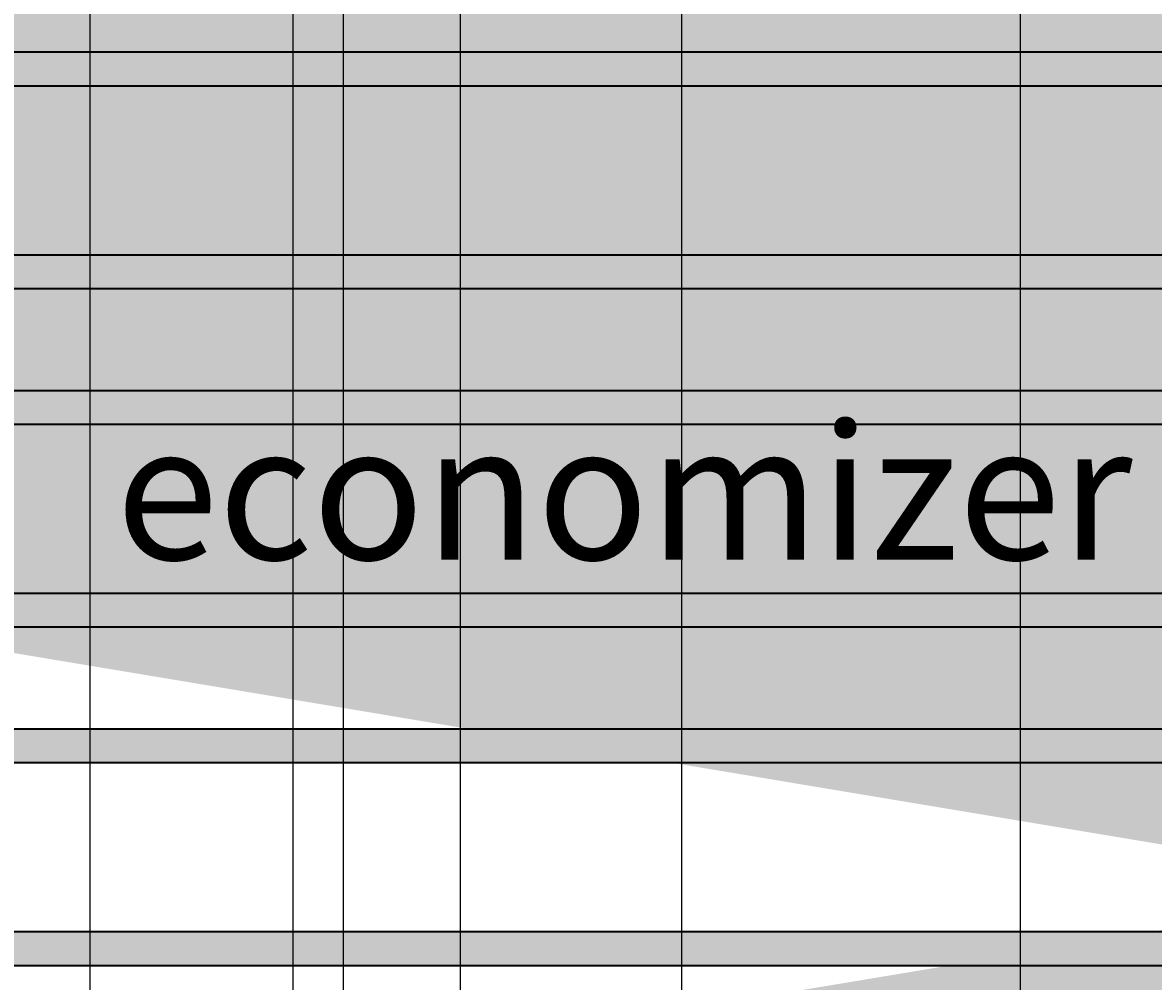
# Model space of a CAD drawing. Units: millimetres. Extents: x -22994 to 29398, y -19990 to 20176.
# Tile 46 of 135: x 136 to 170, y 96 to 124. Entities that reach past the tile are written whole.
import ezdxf

# ---------------------------------------------------------------- set-up
doc = ezdxf.new("R2010")
doc.units = ezdxf.units.MM
doc.header["$MEASUREMENT"] = 0
for name, color, linetype, lineweight in [('M-ANNO-TEXT', 7, 'Continuous', 25), ('M-DIMS', 2, 'Continuous', 18), ('M-EQPM-PATT', 7, 'Continuous', 18), ('M-PIPE', 7, 'Continuous', 35)]:
    doc.layers.add(name, color=color, linetype=linetype, lineweight=lineweight)
doc.styles.get("Standard").update_dxf_attribs({"font": 'arial.ttf'})
doc.dimstyles.get("Standard").update_dxf_attribs({"dimtxt": 0.18, "dimasz": 10000, "dimexe": 0.18, "dimexo": 0.0625, "dimgap": 0.09, "dimtad": 0, "dimtih": 1, "dimtoh": 1, "dimdec": 0, "dimzin": 0, "dimdsep": 46, "dimtxsty": 'Standard', "dimcen": 0.09, "dimadec": 0, "dimazin": 0, "dimtfac": 1, "dimtdec": 0, "dimtofl": 0, "dimtmove": 0, "dimatfit": 3, "dimfxl": 1, "dimtolj": 1, "dimtzin": 0, "dimlwd": 30, "dimarcsym": 0})

# ---------------------------------------------------------------- blocks, each defined once
blk = doc.blocks.new('*D2')
at = {"layer": 'Defpoints', "color": 0, "transparency": 16777216}
for p in [(6.677, 10.271), (290.852, 10.271), (290.852, -5.079)]:
    blk.add_point(p, dxfattribs=at)
at = {"layer": 'M-DIMS', "color": 0, "lineweight": -2, "transparency": 16777216}
for p, q in [((6.677, 10.209), (6.677, -5.259)), ((290.852, 10.209), (290.852, -5.259))]:
    blk.add_line(p, q, dxfattribs=at)
at = {"layer": 'M-DIMS', "color": 0, "lineweight": 30, "transparency": 16777216}
for p, q in [((-9993.323, -5.079), (-19993.323, -5.079)), ((10290.852, -5.079), (20290.852, -5.079))]:
    blk.add_line(p, q, dxfattribs=at)
at = {"layer": 'M-DIMS', "color": 0, "transparency": 16777216}
for points in [[(-9993.323, 1661.588), (-9993.323, -1671.745), (6.677, -5.079)], [(10290.852, 1661.588), (10290.852, -1671.745), (290.852, -5.079)]]:
    blk.add_solid(points, dxfattribs=at)
at = {"layer": 'M-DIMS', "color": 0, "transparency": 16777216, "insert": (148.765, -5.079), "char_height": 0.18, "attachment_point": 5}
blk.add_mtext('\\A1;284.2', dxfattribs=at)
blk = doc.blocks.new('*D3')
at = {"layer": 'Defpoints', "color": 0, "transparency": 16777216}
for p in [(110.265, 204.165), (110.265, 176.366), (95.833, 127.967)]:
    blk.add_point(p, dxfattribs=at)
at = {"layer": 'M-DIMS', "color": 0, "lineweight": -2, "transparency": 16777216}
for p, q in [((95.833, 128.03), (95.833, 204.345)), ((110.265, 176.429), (110.265, 204.345))]:
    blk.add_line(p, q, dxfattribs=at)
at = {"layer": 'M-DIMS', "color": 0, "lineweight": 30, "transparency": 16777216}
for p, q in [((-9904.167, 204.165), (-19904.167, 204.165)), ((10110.265, 204.165), (20110.265, 204.165))]:
    blk.add_line(p, q, dxfattribs=at)
at = {"layer": 'M-DIMS', "color": 0, "transparency": 16777216}
for points in [[(-9904.167, 1870.832), (-9904.167, -1462.501), (95.833, 204.165)], [(10110.265, 1870.832), (10110.265, -1462.501), (110.265, 204.165)]]:
    blk.add_solid(points, dxfattribs=at)
at = {"layer": 'M-DIMS', "color": 0, "transparency": 16777216, "insert": (103.049, 204.165), "char_height": 0.18, "attachment_point": 5}
blk.add_mtext('\\A1;14.432', dxfattribs=at)
blk = doc.blocks.new('*D4')
at = {"layer": 'Defpoints', "color": 0, "transparency": 16777216}
for p in [(116.265, 204.165), (110.265, 176.366), (116.265, 176.366)]:
    blk.add_point(p, dxfattribs=at)
at = {"layer": 'M-DIMS', "color": 0, "lineweight": -2, "transparency": 16777216}
for p, q in [((110.265, 176.429), (110.265, 204.345)), ((116.265, 176.429), (116.265, 204.345))]:
    blk.add_line(p, q, dxfattribs=at)
at = {"layer": 'M-DIMS', "color": 0, "lineweight": 30, "transparency": 16777216}
for p, q in [((-9889.735, 204.165), (-19889.735, 204.165)), ((10116.265, 204.165), (20116.265, 204.165))]:
    blk.add_line(p, q, dxfattribs=at)
at = {"layer": 'M-DIMS', "color": 0, "transparency": 16777216}
for points in [[(-9889.735, 1870.832), (-9889.735, -1462.501), (110.265, 204.165)], [(10116.265, 1870.832), (10116.265, -1462.501), (116.265, 204.165)]]:
    blk.add_solid(points, dxfattribs=at)
at = {"layer": 'M-DIMS', "color": 0, "transparency": 16777216, "insert": (113.265, 204.165), "char_height": 0.18, "attachment_point": 5}
blk.add_mtext('\\A1;6', dxfattribs=at)
blk = doc.blocks.new('*D5')
at = {"layer": 'Defpoints', "color": 0, "transparency": 16777216}
for p in [(181.265, 204.165), (116.265, 176.366), (181.265, 176.366)]:
    blk.add_point(p, dxfattribs=at)
at = {"layer": 'M-DIMS', "color": 0, "lineweight": -2, "transparency": 16777216}
for p, q in [((116.265, 176.429), (116.265, 204.345)), ((181.265, 176.429), (181.265, 204.345))]:
    blk.add_line(p, q, dxfattribs=at)
at = {"layer": 'M-DIMS', "color": 0, "lineweight": 30, "transparency": 16777216}
for p, q in [((-9883.735, 204.165), (-19883.735, 204.165)), ((10181.265, 204.165), (20181.265, 204.165))]:
    blk.add_line(p, q, dxfattribs=at)
at = {"layer": 'M-DIMS', "color": 0, "transparency": 16777216}
for points in [[(-9883.735, 1870.832), (-9883.735, -1462.501), (116.265, 204.165)], [(10181.265, 1870.832), (10181.265, -1462.501), (181.265, 204.165)]]:
    blk.add_solid(points, dxfattribs=at)
at = {"layer": 'M-DIMS', "color": 0, "transparency": 16777216, "insert": (148.765, 204.165), "char_height": 0.18, "attachment_point": 5}
blk.add_mtext('\\A1;65', dxfattribs=at)
blk = doc.blocks.new('*D6')
at = {"layer": 'Defpoints', "color": 0, "transparency": 16777216}
for p in [(187.265, 204.165), (181.265, 176.366), (187.265, 176.366)]:
    blk.add_point(p, dxfattribs=at)
at = {"layer": 'M-DIMS', "color": 0, "lineweight": -2, "transparency": 16777216}
for p, q in [((181.265, 176.429), (181.265, 204.345)), ((187.265, 176.429), (187.265, 204.345))]:
    blk.add_line(p, q, dxfattribs=at)
at = {"layer": 'M-DIMS', "color": 0, "lineweight": 30, "transparency": 16777216}
for p, q in [((-9818.735, 204.165), (-19818.735, 204.165)), ((10187.265, 204.165), (20187.265, 204.165))]:
    blk.add_line(p, q, dxfattribs=at)
at = {"layer": 'M-DIMS', "color": 0, "transparency": 16777216}
for points in [[(-9818.735, 1870.832), (-9818.735, -1462.501), (181.265, 204.165)], [(10187.265, 1870.832), (10187.265, -1462.501), (187.265, 204.165)]]:
    blk.add_solid(points, dxfattribs=at)
at = {"layer": 'M-DIMS', "color": 0, "transparency": 16777216, "insert": (184.265, 204.165), "char_height": 0.18, "attachment_point": 5}
blk.add_mtext('\\A1;6', dxfattribs=at)
blk = doc.blocks.new('*D7')
at = {"layer": 'Defpoints', "color": 0, "transparency": 16777216}
for p in [(201.697, 204.165), (187.265, 176.366), (201.697, 127.967)]:
    blk.add_point(p, dxfattribs=at)
at = {"layer": 'M-DIMS', "color": 0, "lineweight": -2, "transparency": 16777216}
for p, q in [((187.265, 176.429), (187.265, 204.345)), ((201.697, 128.03), (201.697, 204.345))]:
    blk.add_line(p, q, dxfattribs=at)
at = {"layer": 'M-DIMS', "color": 0, "lineweight": 30, "transparency": 16777216}
for p, q in [((-9812.735, 204.165), (-19812.735, 204.165)), ((10201.697, 204.165), (20201.697, 204.165))]:
    blk.add_line(p, q, dxfattribs=at)
at = {"layer": 'M-DIMS', "color": 0, "transparency": 16777216}
for points in [[(-9812.735, 1870.832), (-9812.735, -1462.501), (187.265, 204.165)], [(10201.697, 1870.832), (10201.697, -1462.501), (201.697, 204.165)]]:
    blk.add_solid(points, dxfattribs=at)
at = {"layer": 'M-DIMS', "color": 0, "transparency": 16777216, "insert": (194.481, 204.165), "char_height": 0.18, "attachment_point": 5}
blk.add_mtext('\\A1;14.432', dxfattribs=at)
blk = doc.blocks.new('*D8')
at = {"layer": 'Defpoints', "color": 0, "transparency": 16777216}
for p in [(227.648, 204.165), (227.648, 146.73), (201.697, 127.967)]:
    blk.add_point(p, dxfattribs=at)
at = {"layer": 'M-DIMS', "color": 0, "lineweight": -2, "transparency": 16777216}
for p, q in [((201.697, 128.03), (201.697, 204.345)), ((227.648, 146.792), (227.648, 204.345))]:
    blk.add_line(p, q, dxfattribs=at)
at = {"layer": 'M-DIMS', "color": 0, "lineweight": 30, "transparency": 16777216}
for p, q in [((-9798.303, 204.165), (-19798.303, 204.165)), ((10227.648, 204.165), (20227.648, 204.165))]:
    blk.add_line(p, q, dxfattribs=at)
at = {"layer": 'M-DIMS', "color": 0, "transparency": 16777216}
for points in [[(-9798.303, 1870.832), (-9798.303, -1462.501), (201.697, 204.165)], [(10227.648, 1870.832), (10227.648, -1462.501), (227.648, 204.165)]]:
    blk.add_solid(points, dxfattribs=at)
at = {"layer": 'M-DIMS', "color": 0, "transparency": 16777216, "insert": (214.673, 204.165), "char_height": 0.18, "attachment_point": 5}
blk.add_mtext('\\A1;25.95', dxfattribs=at)
blk = doc.blocks.new('*D9')
at = {"layer": 'Defpoints', "color": 0, "transparency": 16777216}
for p in [(187.265, 176.366), (306.202, 176.366), (290.852, 10.271)]:
    blk.add_point(p, dxfattribs=at)
at = {"layer": 'M-DIMS', "color": 0, "lineweight": 30, "transparency": 16777216}
for p, q in [((306.202, 10176.366), (306.202, 20176.366)), ((306.202, -9989.729), (306.202, -19989.729))]:
    blk.add_line(p, q, dxfattribs=at)
at = {"layer": 'M-DIMS', "color": 0, "lineweight": -2, "transparency": 16777216}
for p, q in [((187.327, 176.366), (306.382, 176.366)), ((290.915, 10.271), (306.382, 10.271))]:
    blk.add_line(p, q, dxfattribs=at)
at = {"layer": 'M-DIMS', "color": 0, "transparency": 16777216}
for points in [[(-1360.465, 10176.366), (1972.869, 10176.366), (306.202, 176.366)], [(-1360.465, -9989.729), (1972.869, -9989.729), (306.202, 10.271)]]:
    blk.add_solid(points, dxfattribs=at)
at = {"layer": 'M-DIMS', "color": 0, "transparency": 16777216, "insert": (306.202, 93.319), "char_height": 0.18, "attachment_point": 5}
blk.add_mtext('\\A1;166.1', dxfattribs=at)
blk = doc.blocks.new('*D10')
at = {"layer": 'Defpoints', "color": 0, "transparency": 16777216}
for p in [(125.65, 136.071), (133.346, 136.071), (133.346, -5.079)]:
    blk.add_point(p, dxfattribs=at)
at = {"layer": 'M-DIMS', "color": 0, "lineweight": -2, "transparency": 16777216}
for p, q in [((125.65, 136.009), (125.65, -5.259)), ((133.346, 136.009), (133.346, -5.259))]:
    blk.add_line(p, q, dxfattribs=at)
at = {"layer": 'M-DIMS', "color": 0, "lineweight": 30, "transparency": 16777216}
for p, q in [((-9874.35, -5.079), (-19874.35, -5.079)), ((10133.346, -5.079), (20133.346, -5.079))]:
    blk.add_line(p, q, dxfattribs=at)
at = {"layer": 'M-DIMS', "color": 0, "transparency": 16777216}
for points in [[(-9874.35, 1661.588), (-9874.35, -1671.745), (125.65, -5.079)], [(10133.346, 1661.588), (10133.346, -1671.745), (133.346, -5.079)]]:
    blk.add_solid(points, dxfattribs=at)
at = {"layer": 'M-DIMS', "color": 0, "transparency": 16777216, "insert": (129.498, -5.079), "char_height": 0.18, "attachment_point": 5}
blk.add_mtext('\\A1;7.696', dxfattribs=at)
blk = doc.blocks.new('*D11')
at = {"layer": 'Defpoints', "color": 0, "transparency": 16777216}
for p in [(133.346, 136.071), (135.65, 136.071), (135.65, -5.079)]:
    blk.add_point(p, dxfattribs=at)
at = {"layer": 'M-DIMS', "color": 0, "lineweight": -2, "transparency": 16777216}
for p, q in [((133.346, 136.009), (133.346, -5.259)), ((135.65, 136.009), (135.65, -5.259))]:
    blk.add_line(p, q, dxfattribs=at)
at = {"layer": 'M-DIMS', "color": 0, "lineweight": 30, "transparency": 16777216}
for p, q in [((-9866.654, -5.079), (-19866.654, -5.079)), ((10135.65, -5.079), (20135.65, -5.079))]:
    blk.add_line(p, q, dxfattribs=at)
at = {"layer": 'M-DIMS', "color": 0, "transparency": 16777216}
for points in [[(-9866.654, 1661.588), (-9866.654, -1671.745), (133.346, -5.079)], [(10135.65, 1661.588), (10135.65, -1671.745), (135.65, -5.079)]]:
    blk.add_solid(points, dxfattribs=at)
at = {"layer": 'M-DIMS', "color": 0, "transparency": 16777216, "insert": (134.498, -5.079), "char_height": 0.18, "attachment_point": 5}
blk.add_mtext('\\A1;2.304', dxfattribs=at)
blk = doc.blocks.new('*D12')
at = {"layer": 'Defpoints', "color": 0, "transparency": 16777216}
for p in [(135.65, 136.071), (145.65, 136.071), (145.65, -5.079)]:
    blk.add_point(p, dxfattribs=at)
at = {"layer": 'M-DIMS', "color": 0, "lineweight": -2, "transparency": 16777216}
for p, q in [((135.65, 136.009), (135.65, -5.259)), ((145.65, 136.009), (145.65, -5.259))]:
    blk.add_line(p, q, dxfattribs=at)
at = {"layer": 'M-DIMS', "color": 0, "lineweight": 30, "transparency": 16777216}
for p, q in [((-9864.35, -5.079), (-19864.35, -5.079)), ((10145.65, -5.079), (20145.65, -5.079))]:
    blk.add_line(p, q, dxfattribs=at)
at = {"layer": 'M-DIMS', "color": 0, "transparency": 16777216}
for points in [[(-9864.35, 1661.588), (-9864.35, -1671.745), (135.65, -5.079)], [(10145.65, 1661.588), (10145.65, -1671.745), (145.65, -5.079)]]:
    blk.add_solid(points, dxfattribs=at)
at = {"layer": 'M-DIMS', "color": 0, "transparency": 16777216, "insert": (140.65, -5.079), "char_height": 0.18, "attachment_point": 5}
blk.add_mtext('\\A1;10', dxfattribs=at)
blk = doc.blocks.new('*D13')
at = {"layer": 'Defpoints', "color": 0, "transparency": 16777216}
for p in [(145.65, 136.071), (155.65, 136.071), (155.65, -5.079)]:
    blk.add_point(p, dxfattribs=at)
at = {"layer": 'M-DIMS', "color": 0, "lineweight": -2, "transparency": 16777216}
for p, q in [((145.65, 136.009), (145.65, -5.259)), ((155.65, 136.009), (155.65, -5.259))]:
    blk.add_line(p, q, dxfattribs=at)
at = {"layer": 'M-DIMS', "color": 0, "lineweight": 30, "transparency": 16777216}
for p, q in [((-9854.35, -5.079), (-19854.35, -5.079)), ((10155.65, -5.079), (20155.65, -5.079))]:
    blk.add_line(p, q, dxfattribs=at)
at = {"layer": 'M-DIMS', "color": 0, "transparency": 16777216}
for points in [[(-9854.35, 1661.588), (-9854.35, -1671.745), (145.65, -5.079)], [(10155.65, 1661.588), (10155.65, -1671.745), (155.65, -5.079)]]:
    blk.add_solid(points, dxfattribs=at)
at = {"layer": 'M-DIMS', "color": 0, "transparency": 16777216, "insert": (150.65, -5.079), "char_height": 0.18, "attachment_point": 5}
blk.add_mtext('\\A1;10', dxfattribs=at)
blk = doc.blocks.new('*D14')
at = {"layer": 'Defpoints', "color": 0, "transparency": 16777216}
for p in [(155.65, 136.071), (165.65, 136.071), (165.65, -5.079)]:
    blk.add_point(p, dxfattribs=at)
at = {"layer": 'M-DIMS', "color": 0, "lineweight": -2, "transparency": 16777216}
for p, q in [((155.65, 136.009), (155.65, -5.259)), ((165.65, 136.009), (165.65, -5.259))]:
    blk.add_line(p, q, dxfattribs=at)
at = {"layer": 'M-DIMS', "color": 0, "lineweight": 30, "transparency": 16777216}
for p, q in [((-9844.35, -5.079), (-19844.35, -5.079)), ((10165.65, -5.079), (20165.65, -5.079))]:
    blk.add_line(p, q, dxfattribs=at)
at = {"layer": 'M-DIMS', "color": 0, "transparency": 16777216}
for points in [[(-9844.35, 1661.588), (-9844.35, -1671.745), (155.65, -5.079)], [(10165.65, 1661.588), (10165.65, -1671.745), (165.65, -5.079)]]:
    blk.add_solid(points, dxfattribs=at)
at = {"layer": 'M-DIMS', "color": 0, "transparency": 16777216, "insert": (160.65, -5.079), "char_height": 0.18, "attachment_point": 5}
blk.add_mtext('\\A1;10', dxfattribs=at)
blk = doc.blocks.new('*D15')
at = {"layer": 'Defpoints', "color": 0, "transparency": 16777216}
for p in [(173.346, 154.788), (173.346, 136.071), (306.202, 136.071)]:
    blk.add_point(p, dxfattribs=at)
at = {"layer": 'M-DIMS', "color": 0, "lineweight": 30, "transparency": 16777216}
for p, q in [((306.202, 10154.788), (306.202, 20154.788)), ((306.202, -9863.929), (306.202, -19863.929))]:
    blk.add_line(p, q, dxfattribs=at)
at = {"layer": 'M-DIMS', "color": 0, "lineweight": -2, "transparency": 16777216}
for p, q in [((173.408, 154.788), (306.382, 154.788)), ((173.408, 136.071), (306.382, 136.071))]:
    blk.add_line(p, q, dxfattribs=at)
at = {"layer": 'M-DIMS', "color": 0, "transparency": 16777216}
for points in [[(-1360.465, 10154.788), (1972.869, 10154.788), (306.202, 154.788)], [(-1360.465, -9863.929), (1972.869, -9863.929), (306.202, 136.071)]]:
    blk.add_solid(points, dxfattribs=at)
at = {"layer": 'M-DIMS', "color": 0, "transparency": 16777216, "insert": (306.202, 145.43), "char_height": 0.18, "attachment_point": 5}
blk.add_mtext('\\A1;18.717', dxfattribs=at)
blk = doc.blocks.new('*D16')
at = {"layer": 'Defpoints', "color": 0, "transparency": 16777216}
for p in [(120.17, 204.165), (110.466, 48.035), (120.17, 48.035)]:
    blk.add_point(p, dxfattribs=at)
at = {"layer": 'M-DIMS', "color": 0, "lineweight": -2, "transparency": 16777216}
for p, q in [((110.466, 48.097), (110.466, 204.345)), ((120.17, 48.097), (120.17, 204.345))]:
    blk.add_line(p, q, dxfattribs=at)
at = {"layer": 'M-DIMS', "color": 0, "lineweight": 30, "transparency": 16777216}
for p, q in [((-9889.534, 204.165), (-19889.534, 204.165)), ((10120.17, 204.165), (20120.17, 204.165))]:
    blk.add_line(p, q, dxfattribs=at)
at = {"layer": 'M-DIMS', "color": 0, "transparency": 16777216}
for points in [[(-9889.534, 1870.832), (-9889.534, -1462.501), (110.466, 204.165)], [(10120.17, 1870.832), (10120.17, -1462.501), (120.17, 204.165)]]:
    blk.add_solid(points, dxfattribs=at)
at = {"layer": 'M-DIMS', "color": 0, "transparency": 16777216, "insert": (115.318, 204.165), "char_height": 0.18, "attachment_point": 5}
blk.add_mtext('\\A1;9.704', dxfattribs=at)
blk = doc.blocks.new('*D17')
at = {"layer": 'Defpoints', "color": 0, "transparency": 16777216}
for p in [(126.17, 204.165), (120.17, 48.035), (126.17, 48.035)]:
    blk.add_point(p, dxfattribs=at)
at = {"layer": 'M-DIMS', "color": 0, "lineweight": -2, "transparency": 16777216}
for p, q in [((120.17, 48.097), (120.17, 204.345)), ((126.17, 48.097), (126.17, 204.345))]:
    blk.add_line(p, q, dxfattribs=at)
at = {"layer": 'M-DIMS', "color": 0, "lineweight": 30, "transparency": 16777216}
for p, q in [((-9879.83, 204.165), (-19879.83, 204.165)), ((10126.17, 204.165), (20126.17, 204.165))]:
    blk.add_line(p, q, dxfattribs=at)
at = {"layer": 'M-DIMS', "color": 0, "transparency": 16777216}
for points in [[(-9879.83, 1870.832), (-9879.83, -1462.501), (120.17, 204.165)], [(10126.17, 1870.832), (10126.17, -1462.501), (126.17, 204.165)]]:
    blk.add_solid(points, dxfattribs=at)
at = {"layer": 'M-DIMS', "color": 0, "transparency": 16777216, "insert": (123.17, 204.165), "char_height": 0.18, "attachment_point": 5}
blk.add_mtext('\\A1;6', dxfattribs=at)
blk = doc.blocks.new('*D18')
at = {"layer": 'Defpoints', "color": 0, "transparency": 16777216}
for p in [(132.17, 204.165), (126.17, 48.035), (132.17, 48.035)]:
    blk.add_point(p, dxfattribs=at)
at = {"layer": 'M-DIMS', "color": 0, "lineweight": -2, "transparency": 16777216}
for p, q in [((126.17, 48.097), (126.17, 204.345)), ((132.17, 48.097), (132.17, 204.345))]:
    blk.add_line(p, q, dxfattribs=at)
at = {"layer": 'M-DIMS', "color": 0, "lineweight": 30, "transparency": 16777216}
for p, q in [((-9873.83, 204.165), (-19873.83, 204.165)), ((10132.17, 204.165), (20132.17, 204.165))]:
    blk.add_line(p, q, dxfattribs=at)
at = {"layer": 'M-DIMS', "color": 0, "transparency": 16777216}
for points in [[(-9873.83, 1870.832), (-9873.83, -1462.501), (126.17, 204.165)], [(10132.17, 1870.832), (10132.17, -1462.501), (132.17, 204.165)]]:
    blk.add_solid(points, dxfattribs=at)
at = {"layer": 'M-DIMS', "color": 0, "transparency": 16777216, "insert": (129.17, 204.165), "char_height": 0.18, "attachment_point": 5}
blk.add_mtext('\\A1;6', dxfattribs=at)
blk = doc.blocks.new('*D19')
at = {"layer": 'Defpoints', "color": 0, "transparency": 16777216}
for p in [(138.17, 204.165), (132.17, 48.035), (138.17, 48.035)]:
    blk.add_point(p, dxfattribs=at)
at = {"layer": 'M-DIMS', "color": 0, "lineweight": -2, "transparency": 16777216}
for p, q in [((132.17, 48.097), (132.17, 204.345)), ((138.17, 48.097), (138.17, 204.345))]:
    blk.add_line(p, q, dxfattribs=at)
at = {"layer": 'M-DIMS', "color": 0, "lineweight": 30, "transparency": 16777216}
for p, q in [((-9867.83, 204.165), (-19867.83, 204.165)), ((10138.17, 204.165), (20138.17, 204.165))]:
    blk.add_line(p, q, dxfattribs=at)
at = {"layer": 'M-DIMS', "color": 0, "transparency": 16777216}
for points in [[(-9867.83, 1870.832), (-9867.83, -1462.501), (132.17, 204.165)], [(10138.17, 1870.832), (10138.17, -1462.501), (138.17, 204.165)]]:
    blk.add_solid(points, dxfattribs=at)
at = {"layer": 'M-DIMS', "color": 0, "transparency": 16777216, "insert": (135.17, 204.165), "char_height": 0.18, "attachment_point": 5}
blk.add_mtext('\\A1;6', dxfattribs=at)
blk = doc.blocks.new('*D20')
at = {"layer": 'Defpoints', "color": 0, "transparency": 16777216}
for p in [(144.17, 204.165), (138.17, 48.035), (144.17, 48.035)]:
    blk.add_point(p, dxfattribs=at)
at = {"layer": 'M-DIMS', "color": 0, "lineweight": -2, "transparency": 16777216}
for p, q in [((138.17, 48.097), (138.17, 204.345)), ((144.17, 48.097), (144.17, 204.345))]:
    blk.add_line(p, q, dxfattribs=at)
at = {"layer": 'M-DIMS', "color": 0, "lineweight": 30, "transparency": 16777216}
for p, q in [((-9861.83, 204.165), (-19861.83, 204.165)), ((10144.17, 204.165), (20144.17, 204.165))]:
    blk.add_line(p, q, dxfattribs=at)
at = {"layer": 'M-DIMS', "color": 0, "transparency": 16777216}
for points in [[(-9861.83, 1870.832), (-9861.83, -1462.501), (138.17, 204.165)], [(10144.17, 1870.832), (10144.17, -1462.501), (144.17, 204.165)]]:
    blk.add_solid(points, dxfattribs=at)
at = {"layer": 'M-DIMS', "color": 0, "transparency": 16777216, "insert": (141.17, 204.165), "char_height": 0.18, "attachment_point": 5}
blk.add_mtext('\\A1;6', dxfattribs=at)
blk = doc.blocks.new('*D21')
at = {"layer": 'Defpoints', "color": 0, "transparency": 16777216}
for p in [(149.116, 204.165), (144.17, 48.035), (149.116, 48.035)]:
    blk.add_point(p, dxfattribs=at)
at = {"layer": 'M-DIMS', "color": 0, "lineweight": -2, "transparency": 16777216}
for p, q in [((144.17, 48.097), (144.17, 204.345)), ((149.116, 48.097), (149.116, 204.345))]:
    blk.add_line(p, q, dxfattribs=at)
at = {"layer": 'M-DIMS', "color": 0, "lineweight": 30, "transparency": 16777216}
for p, q in [((-9855.83, 204.165), (-19855.83, 204.165)), ((10149.116, 204.165), (20149.116, 204.165))]:
    blk.add_line(p, q, dxfattribs=at)
at = {"layer": 'M-DIMS', "color": 0, "transparency": 16777216}
for points in [[(-9855.83, 1870.832), (-9855.83, -1462.501), (144.17, 204.165)], [(10149.116, 1870.832), (10149.116, -1462.501), (149.116, 204.165)]]:
    blk.add_solid(points, dxfattribs=at)
at = {"layer": 'M-DIMS', "color": 0, "transparency": 16777216, "insert": (146.643, 204.165), "char_height": 0.18, "attachment_point": 5}
blk.add_mtext('\\A1;4.945', dxfattribs=at)
blk = doc.blocks.new('*D22')
at = {"layer": 'Defpoints', "color": 0, "transparency": 16777216}
for p in [(149.116, 30.99), (155.116, 30.99), (155.116, -5.079)]:
    blk.add_point(p, dxfattribs=at)
at = {"layer": 'M-DIMS', "color": 0, "lineweight": -2, "transparency": 16777216}
for p, q in [((149.116, 30.927), (149.116, -5.259)), ((155.116, 30.927), (155.116, -5.259))]:
    blk.add_line(p, q, dxfattribs=at)
at = {"layer": 'M-DIMS', "color": 0, "lineweight": 30, "transparency": 16777216}
for p, q in [((-9850.884, -5.079), (-19850.884, -5.079)), ((10155.116, -5.079), (20155.116, -5.079))]:
    blk.add_line(p, q, dxfattribs=at)
at = {"layer": 'M-DIMS', "color": 0, "transparency": 16777216}
for points in [[(-9850.884, 1661.588), (-9850.884, -1671.745), (149.116, -5.079)], [(10155.116, 1661.588), (10155.116, -1671.745), (155.116, -5.079)]]:
    blk.add_solid(points, dxfattribs=at)
at = {"layer": 'M-DIMS', "color": 0, "transparency": 16777216, "insert": (152.116, -5.079), "char_height": 0.18, "attachment_point": 5}
blk.add_mtext('\\A1;6', dxfattribs=at)
blk = doc.blocks.new('*D23')
at = {"layer": 'Defpoints', "color": 0, "transparency": 16777216}
for p in [(155.116, 30.99), (161.116, 30.99), (161.116, -5.079)]:
    blk.add_point(p, dxfattribs=at)
at = {"layer": 'M-DIMS', "color": 0, "lineweight": -2, "transparency": 16777216}
for p, q in [((155.116, 30.927), (155.116, -5.259)), ((161.116, 30.927), (161.116, -5.259))]:
    blk.add_line(p, q, dxfattribs=at)
at = {"layer": 'M-DIMS', "color": 0, "lineweight": 30, "transparency": 16777216}
for p, q in [((-9844.884, -5.079), (-19844.884, -5.079)), ((10161.116, -5.079), (20161.116, -5.079))]:
    blk.add_line(p, q, dxfattribs=at)
at = {"layer": 'M-DIMS', "color": 0, "transparency": 16777216}
for points in [[(-9844.884, 1661.588), (-9844.884, -1671.745), (155.116, -5.079)], [(10161.116, 1661.588), (10161.116, -1671.745), (161.116, -5.079)]]:
    blk.add_solid(points, dxfattribs=at)
at = {"layer": 'M-DIMS', "color": 0, "transparency": 16777216, "insert": (158.116, -5.079), "char_height": 0.18, "attachment_point": 5}
blk.add_mtext('\\A1;6', dxfattribs=at)
blk = doc.blocks.new('*D24')
at = {"layer": 'Defpoints', "color": 0, "transparency": 16777216}
for p in [(161.116, 30.99), (166.439, 30.99), (166.439, -5.079)]:
    blk.add_point(p, dxfattribs=at)
at = {"layer": 'M-DIMS', "color": 0, "lineweight": -2, "transparency": 16777216}
for p, q in [((161.116, 30.927), (161.116, -5.259)), ((166.439, 30.927), (166.439, -5.259))]:
    blk.add_line(p, q, dxfattribs=at)
at = {"layer": 'M-DIMS', "color": 0, "lineweight": 30, "transparency": 16777216}
for p, q in [((-9838.884, -5.079), (-19838.884, -5.079)), ((10166.439, -5.079), (20166.439, -5.079))]:
    blk.add_line(p, q, dxfattribs=at)
at = {"layer": 'M-DIMS', "color": 0, "transparency": 16777216}
for points in [[(-9838.884, 1661.588), (-9838.884, -1671.745), (161.116, -5.079)], [(10166.439, 1661.588), (10166.439, -1671.745), (166.439, -5.079)]]:
    blk.add_solid(points, dxfattribs=at)
at = {"layer": 'M-DIMS', "color": 0, "transparency": 16777216, "insert": (163.777, -5.079), "char_height": 0.18, "attachment_point": 5}
blk.add_mtext('\\A1;5.323', dxfattribs=at)
blk = doc.blocks.new('*D25')
at = {"layer": 'Defpoints', "color": 0, "transparency": 16777216}
for p in [(166.439, 30.99), (172.439, 30.99), (172.439, -5.079)]:
    blk.add_point(p, dxfattribs=at)
at = {"layer": 'M-DIMS', "color": 0, "lineweight": -2, "transparency": 16777216}
for p, q in [((166.439, 30.927), (166.439, -5.259)), ((172.439, 30.927), (172.439, -5.259))]:
    blk.add_line(p, q, dxfattribs=at)
at = {"layer": 'M-DIMS', "color": 0, "lineweight": 30, "transparency": 16777216}
for p, q in [((-9833.561, -5.079), (-19833.561, -5.079)), ((10172.439, -5.079), (20172.439, -5.079))]:
    blk.add_line(p, q, dxfattribs=at)
at = {"layer": 'M-DIMS', "color": 0, "transparency": 16777216}
for points in [[(-9833.561, 1661.588), (-9833.561, -1671.745), (166.439, -5.079)], [(10172.439, 1661.588), (10172.439, -1671.745), (172.439, -5.079)]]:
    blk.add_solid(points, dxfattribs=at)
at = {"layer": 'M-DIMS', "color": 0, "transparency": 16777216, "insert": (169.439, -5.079), "char_height": 0.18, "attachment_point": 5}
blk.add_mtext('\\A1;6', dxfattribs=at)
blk = doc.blocks.new('*D26')
at = {"layer": 'Defpoints', "color": 0, "transparency": 16777216}
for p in [(172.439, 30.99), (178.439, 30.99), (178.439, -5.079)]:
    blk.add_point(p, dxfattribs=at)
at = {"layer": 'M-DIMS', "color": 0, "lineweight": -2, "transparency": 16777216}
for p, q in [((172.439, 30.927), (172.439, -5.259)), ((178.439, 30.927), (178.439, -5.259))]:
    blk.add_line(p, q, dxfattribs=at)
at = {"layer": 'M-DIMS', "color": 0, "lineweight": 30, "transparency": 16777216}
for p, q in [((-9827.561, -5.079), (-19827.561, -5.079)), ((10178.439, -5.079), (20178.439, -5.079))]:
    blk.add_line(p, q, dxfattribs=at)
at = {"layer": 'M-DIMS', "color": 0, "transparency": 16777216}
for points in [[(-9827.561, 1661.588), (-9827.561, -1671.745), (172.439, -5.079)], [(10178.439, 1661.588), (10178.439, -1671.745), (178.439, -5.079)]]:
    blk.add_solid(points, dxfattribs=at)
at = {"layer": 'M-DIMS', "color": 0, "transparency": 16777216, "insert": (175.439, -5.079), "char_height": 0.18, "attachment_point": 5}
blk.add_mtext('\\A1;6', dxfattribs=at)
blk = doc.blocks.new('*D27')
at = {"layer": 'Defpoints', "color": 0, "transparency": 16777216}
for p in [(178.439, 30.99), (188.117, 30.99), (188.117, -5.079)]:
    blk.add_point(p, dxfattribs=at)
at = {"layer": 'M-DIMS', "color": 0, "lineweight": -2, "transparency": 16777216}
for p, q in [((178.439, 30.927), (178.439, -5.259)), ((188.117, 30.927), (188.117, -5.259))]:
    blk.add_line(p, q, dxfattribs=at)
at = {"layer": 'M-DIMS', "color": 0, "lineweight": 30, "transparency": 16777216}
for p, q in [((-9821.561, -5.079), (-19821.561, -5.079)), ((10188.117, -5.079), (20188.117, -5.079))]:
    blk.add_line(p, q, dxfattribs=at)
at = {"layer": 'M-DIMS', "color": 0, "transparency": 16777216}
for points in [[(-9821.561, 1661.588), (-9821.561, -1671.745), (178.439, -5.079)], [(10188.117, 1661.588), (10188.117, -1671.745), (188.117, -5.079)]]:
    blk.add_solid(points, dxfattribs=at)
at = {"layer": 'M-DIMS', "color": 0, "transparency": 16777216, "insert": (183.278, -5.079), "char_height": 0.18, "attachment_point": 5}
blk.add_mtext('\\A1;9.679', dxfattribs=at)
blk = doc.blocks.new('*D28')
at = {"layer": 'Defpoints', "color": 0, "transparency": 16777216}
for p in [(188.117, 48.035), (306.202, 48.035), (188.117, 30.99)]:
    blk.add_point(p, dxfattribs=at)
at = {"layer": 'M-DIMS', "color": 0, "lineweight": 30, "transparency": 16777216}
for p, q in [((306.202, 10048.035), (306.202, 20048.035)), ((306.202, -9969.01), (306.202, -19969.01))]:
    blk.add_line(p, q, dxfattribs=at)
at = {"layer": 'M-DIMS', "color": 0, "lineweight": -2, "transparency": 16777216}
for p, q in [((188.18, 48.035), (306.382, 48.035)), ((188.18, 30.99), (306.382, 30.99))]:
    blk.add_line(p, q, dxfattribs=at)
at = {"layer": 'M-DIMS', "color": 0, "transparency": 16777216}
for points in [[(-1360.465, 10048.035), (1972.869, 10048.035), (306.202, 48.035)], [(-1360.465, -9969.01), (1972.869, -9969.01), (306.202, 30.99)]]:
    blk.add_solid(points, dxfattribs=at)
at = {"layer": 'M-DIMS', "color": 0, "transparency": 16777216, "insert": (306.202, 39.512), "char_height": 0.18, "attachment_point": 5}
blk.add_mtext('\\A1;17.045', dxfattribs=at)
blk = doc.blocks.new('*D29')
at = {"layer": 'Defpoints', "color": 0, "transparency": 16777216}
for p in [(36.801, 80.045), (64.03, 80.045)]:
    blk.add_point(p, dxfattribs=at)
at = {"layer": 'M-DIMS', "color": 0, "lineweight": -2, "transparency": 16777216}
for p, q in [((50.325, 80.045), (50.505, 80.045)), ((50.415, 79.955), (50.415, 80.135))]:
    blk.add_line(p, q, dxfattribs=at)
at = {"layer": 'M-DIMS', "color": 0, "lineweight": 30, "transparency": 16777216}
blk.add_line((20064.03, 80.03), (10064.03, 80.038), dxfattribs=at)
at = {"layer": 'M-DIMS', "color": 0, "transparency": 16777216}
blk.add_solid([(10064.031, 1746.704), (10064.028, -1586.629), (64.03, 80.045)], dxfattribs=at)
at = {"layer": 'M-DIMS', "color": 0, "transparency": 16777216, "insert": (20064.521, 80.03), "char_height": 0.18, "attachment_point": 5}
blk.add_mtext('\\A1;∅27.23', dxfattribs=at)
blk = doc.blocks.new('*D36')
at = {"layer": 'Defpoints', "color": 0, "transparency": 16777216}
for p in [(46.39, 31.303), (46.387, 26.593)]:
    blk.add_point(p, dxfattribs=at)
at = {"layer": 'M-DIMS', "color": 0, "lineweight": 30, "transparency": 16777216}
for p, q in [((57.15, 20031.301), (51.77, 10031.302)), ((10057.15, 20031.301), (57.15, 20031.301))]:
    blk.add_line(p, q, dxfattribs=at)
at = {"layer": 'M-DIMS', "color": 0, "lineweight": -2, "transparency": 16777216}
for p, q in [((46.299, 28.948), (46.479, 28.948)), ((46.389, 28.858), (46.389, 29.038))]:
    blk.add_line(p, q, dxfattribs=at)
at = {"layer": 'M-DIMS', "color": 0, "transparency": 16777216}
blk.add_solid([(-1614.896, 10032.199), (1718.436, 10030.405), (46.39, 31.303)], dxfattribs=at)
at = {"layer": 'M-DIMS', "color": 0, "transparency": 16777216, "insert": (10057.554, 20031.301), "char_height": 0.18, "attachment_point": 5}
blk.add_mtext('\\A1;∅4.71', dxfattribs=at)
blk = doc.blocks.new('*D37')
at = {"layer": 'Defpoints', "color": 0, "transparency": 16777216}
for p in [(54.834, 118.615), (59.494, 118.614)]:
    blk.add_point(p, dxfattribs=at)
at = {"layer": 'M-DIMS', "color": 0, "lineweight": -2, "transparency": 16777216}
for p, q in [((57.164, 118.524), (57.164, 118.704)), ((57.074, 118.614), (57.254, 118.614))]:
    blk.add_line(p, q, dxfattribs=at)
at = {"layer": 'M-DIMS', "color": 0, "lineweight": 30, "transparency": 16777216}
blk.add_line((20059.493, 116.253), (10059.494, 117.434), dxfattribs=at)
at = {"layer": 'M-DIMS', "color": 0, "transparency": 16777216}
blk.add_solid([(10059.69, 1784.1), (10059.297, -1549.233), (59.494, 118.614)], dxfattribs=at)
at = {"layer": 'M-DIMS', "color": 0, "transparency": 16777216, "insert": (20059.985, 116.253), "char_height": 0.18, "attachment_point": 5}
blk.add_mtext('\\A1;∅4.659', dxfattribs=at)

msp = doc.modelspace()

# ---------------------------------------------------------------- hatches: boundary and pattern name
at = {"layer": 'M-EQPM-PATT'}
h = msp.add_hatch(color=256, dxfattribs=at)
h.set_gradient(color1=(34, 52, 110), color2=(41, 49, 137), tint=1, name='CYLINDER')
h.paths.add_polyline_path([(101.8327, 123.6277), (101.8327, 122.6277), (176.8123, 122.6277, -0.4142136), (178.3123, 121.1277), (178.3123, 119.1277, -0.4142136), (176.8123, 117.6277), (129.8123, 117.6277, 0.4142136), (128.3123, 116.1277), (128.3123, 114.1277, 0.4142136), (129.8123, 112.6277), (176.8123, 112.6277, -0.4142136), (178.3123, 111.1277), (178.3123, 109.1277, -0.4142136), (176.8123, 107.6277), (129.8123, 107.6277, 0.4142136), (128.3123, 106.1277), (128.3123, 104.1277, 0.4142136), (129.8123, 102.6277), (176.8123, 102.6277, -0.4142136), (178.3123, 101.1277), (178.3123, 99.1277, -0.4142136), (176.8123, 97.6277), (101.8327, 97.6277), (101.8327, 96.6277), (176.8123, 96.6277, 0.4142136), (179.3123, 99.1277), (179.3123, 101.1277, 0.4142136), (176.8123, 103.6277), (129.8123, 103.6277, -0.4142136), (129.3123, 104.1277), (129.3123, 106.1277, -0.4142136), (129.8123, 106.6277), (176.8123, 106.6277, 0.4142136), (179.3123, 109.1277), (179.3123, 111.1277, 0.4142136), (176.8123, 113.6277), (129.8123, 113.6277, -0.4142136), (129.3123, 114.1277), (129.3123, 116.1277, -0.4142136), (129.8123, 116.6277), (176.8123, 116.6277, 0.4142136), (179.3123, 119.1277), (179.3123, 121.1277, 0.4142136), (176.8123, 123.6277)])
h.paths.add_polyline_path([(75.6657, 123.6277), (75.6657, 122.6277), (95.8327, 122.6277), (95.8327, 123.6277)])
h.paths.add_polyline_path([(51.0853, 122.6277, -0.0439182), (51.8797, 123.6277), (38.9157, 123.6277), (38.9157, 122.6277)])
h.paths.add_polyline_path([(95.8327, 96.6277), (95.8327, 97.6277), (22.2694, 97.6277, 0.4142136), (20.7694, 96.1277), (20.7694, 89.8712, 0.4142136), (22.2694, 88.3712), (39.6435, 88.3712, -0.024152), (40.4967, 89.3712), (23.2694, 89.3712, -0.4142136), (21.7694, 90.8712), (21.7694, 95.1277, -0.4142136), (23.2694, 96.6277)])
h.paths.add_polyline_path([(137.7248, 106.4435), (168.6853, 106.4435), (168.6853, 114.6864), (137.7248, 114.6864)], flags=25)

# ---------------------------------------------------------------- linework, layer by layer
at = {"layer": 'M-PIPE'}
for points in [[(101.8327, 123.6277), (176.8123, 123.6277, -0.4142136), (179.3123, 121.1277), (179.3123, 119.1277, -0.4142136), (176.8123, 116.6277), (129.8123, 116.6277, 0.4142136), (129.3123, 116.1277), (129.3123, 114.1277, 0.4142136), (129.8123, 113.6277), (176.8123, 113.6277, -0.4142136), (179.3123, 111.1277), (179.3123, 109.1277, -0.4142136), (176.8123, 106.6277), (129.8123, 106.6277, 0.4142136), (129.3123, 106.1277), (129.3123, 104.1277, 0.4142136), (129.8123, 103.6277), (176.8123, 103.6277, -0.4142136), (179.3123, 101.1277), (179.3123, 99.1277, -0.4142136), (176.8123, 96.6277), (101.8327, 96.6277)], [(101.8327, 122.6277), (176.8123, 122.6277, -0.4142136), (178.3123, 121.1277), (178.3123, 119.1277, -0.4142136), (176.8123, 117.6277), (129.8123, 117.6277, 0.4142136), (128.3123, 116.1277), (128.3123, 114.1277, 0.4142136), (129.8123, 112.6277), (176.8123, 112.6277, -0.4142136), (178.3123, 111.1277), (178.3123, 109.1277, -0.4142136), (176.8123, 107.6277), (129.8123, 107.6277, 0.4142136), (128.3123, 106.1277), (128.3123, 104.1277, 0.4142136), (129.8123, 102.6277), (176.8123, 102.6277, -0.4142136), (178.3123, 101.1277), (178.3123, 99.1277, -0.4142136), (176.8123, 97.6277), (101.8327, 97.6277)]]:
    msp.add_lwpolyline(points, format="xyb", dxfattribs=at)

# ---------------------------------------------------------------- texts
at = {"layer": 'M-ANNO-TEXT', "insert": (138.9295, 112.6277), "char_height": 4, "attachment_point": 1}
msp.add_mtext_dynamic_manual_height_columns('economizer', width=37.883315, gutter_width=1, heights=[0], dxfattribs=at)

# ---------------------------------------------------------------- dimensions: what is measured, and where the dimension line sits
at = {"layer": 'M-DIMS'}
for base, p1, p2, override, picture, middle in [((306.202, 176.3662), (290.852, 10.2713), (187.2647, 176.3662), {"dimdec": 1, "dimlfac": 1, "dimrnd": 0, "dimzin": 0, "dimdsep": 46, "dimlunit": 2}, '*D9', (306.202, 93.3187)), ((306.202, 136.0713), (173.3459, 154.788), (173.3459, 136.0713), {"dimdec": 3, "dimlfac": 1, "dimrnd": 0, "dimzin": 0, "dimdsep": 46, "dimlunit": 2}, '*D15', (306.202, 145.4297)), ((306.202, 48.0349), (188.1175, 30.9895), (188.1175, 48.0349), {"dimdec": 3, "dimlfac": 1, "dimrnd": 0, "dimzin": 0, "dimdsep": 46, "dimlunit": 2}, '*D28', (306.202, 39.5122))]:
    dim = msp.add_linear_dim(base=base, p1=p1, p2=p2, angle=90, dimstyle='Standard', override=override, dxfattribs=at)
    dim.commit()
    dim.dimension.update_dxf_attribs({"geometry": picture, "text_midpoint": middle})
dim = msp.add_diameter_dim_2p(p1=(46.3875, 26.5934), p2=(46.39, 31.3035), dimstyle='Standard', override={"dimdec": 2, "dimlfac": 1, "dimrnd": 0, "dimzin": 0, "dimdsep": 46, "dimlunit": 2}, dxfattribs=at)
dim.commit()
dim.dimension.update_dxf_attribs({"geometry": '*D36', "text_midpoint": (10057.5542, 20031.3006), "dimtype": 163})
for base, p1, p2, override, picture, middle in [((110.2647, 204.1654), (95.8327, 127.967), (110.2647, 176.3662), {"dimdec": 3, "dimlfac": 1, "dimrnd": 0, "dimzin": 0, "dimdsep": 46, "dimlunit": 2}, '*D3', (103.0487, 204.1654)), ((116.2647, 204.1654), (110.2647, 176.3662), (116.2647, 176.3662), {"dimdec": 0, "dimlfac": 1, "dimrnd": 0, "dimzin": 0, "dimdsep": 46, "dimlunit": 2}, '*D4', (113.2647, 204.1654)), ((120.1702, 204.1654), (110.4658, 48.0349), (120.1702, 48.0349), {"dimdec": 3, "dimlfac": 1, "dimrnd": 0, "dimzin": 0, "dimdsep": 46, "dimlunit": 2}, '*D16', (115.318, 204.1654)), ((181.2647, 204.1654), (116.2647, 176.3662), (181.2647, 176.3662), {"dimdec": 0, "dimlfac": 1, "dimrnd": 0, "dimzin": 0, "dimdsep": 46, "dimlunit": 2}, '*D5', (148.7647, 204.1654)), ((126.1702, 204.1654), (120.1702, 48.0349), (126.1702, 48.0349), {"dimdec": 0, "dimlfac": 1, "dimrnd": 0, "dimzin": 0, "dimdsep": 46, "dimlunit": 2}, '*D17', (123.1702, 204.1654)), ((132.1702, 204.1654), (126.1702, 48.0349), (132.1702, 48.0349), {"dimdec": 0, "dimlfac": 1, "dimrnd": 0, "dimzin": 0, "dimdsep": 46, "dimlunit": 2}, '*D18', (129.1702, 204.1654)), ((138.1702, 204.1654), (132.1702, 48.0349), (138.1702, 48.0349), {"dimdec": 0, "dimlfac": 1, "dimrnd": 0, "dimzin": 0, "dimdsep": 46, "dimlunit": 2}, '*D19', (135.1702, 204.1654)), ((144.1702, 204.1654), (138.1702, 48.0349), (144.1702, 48.0349), {"dimdec": 0, "dimlfac": 1, "dimrnd": 0, "dimzin": 0, "dimdsep": 46, "dimlunit": 2}, '*D20', (141.1702, 204.1654)), ((149.11567, 204.16539), (144.17023, 48.03494), (149.11567, 48.03494), {"dimdec": 3, "dimlfac": 1, "dimrnd": 0, "dimzin": 0, "dimdsep": 46, "dimlunit": 2}, '*D21', (146.64295, 204.16539)), ((187.2647, 204.1654), (181.2647, 176.3662), (187.2647, 176.3662), {"dimdec": 0, "dimlfac": 1, "dimrnd": 0, "dimzin": 0, "dimdsep": 46, "dimlunit": 2}, '*D6', (184.2647, 204.1654)), ((201.6967, 204.1654), (187.2647, 176.3662), (201.6967, 127.967), {"dimdec": 3, "dimlfac": 1, "dimrnd": 0, "dimzin": 0, "dimdsep": 46, "dimlunit": 2}, '*D7', (194.4807, 204.1654)), ((227.6485, 204.1654), (201.6967, 127.967), (227.6485, 146.7296), {"dimdec": 2, "dimlfac": 1, "dimrnd": 0, "dimzin": 0, "dimdsep": 46, "dimlunit": 2}, '*D8', (214.6726, 204.1654)), ((290.852, -5.0787), (6.6773, 10.2713), (290.852, 10.2713), {"dimdec": 1, "dimlfac": 1, "dimrnd": 0, "dimzin": 0, "dimdsep": 46, "dimlunit": 2}, '*D2', (148.7647, -5.0787)), ((133.3459, -5.0787), (125.6498, 136.0713), (133.3459, 136.0713), {"dimdec": 3, "dimlfac": 1, "dimrnd": 0, "dimzin": 0, "dimdsep": 46, "dimlunit": 2}, '*D10', (129.4978, -5.0787)), ((135.6498, -5.0787), (133.3459, 136.0713), (135.6498, 136.0713), {"dimdec": 3, "dimlfac": 1, "dimrnd": 0, "dimzin": 0, "dimdsep": 46, "dimlunit": 2}, '*D11', (134.4978, -5.0787)), ((145.6498, -5.0787), (135.6498, 136.0713), (145.6498, 136.0713), {"dimdec": 0, "dimlfac": 1, "dimrnd": 0, "dimzin": 0, "dimdsep": 46, "dimlunit": 2}, '*D12', (140.6498, -5.0787)), ((155.6498, -5.0787), (145.6498, 136.0713), (155.6498, 136.0713), {"dimdec": 0, "dimlfac": 1, "dimrnd": 0, "dimzin": 0, "dimdsep": 46, "dimlunit": 2}, '*D13', (150.6498, -5.0787)), ((155.1157, -5.0787), (149.1157, 30.9895), (155.1157, 30.9895), {"dimdec": 0, "dimlfac": 1, "dimrnd": 0, "dimzin": 0, "dimdsep": 46, "dimlunit": 2}, '*D22', (152.1157, -5.0787)), ((161.1157, -5.0787), (155.1157, 30.9895), (161.1157, 30.9895), {"dimdec": 0, "dimlfac": 1, "dimrnd": 0, "dimzin": 0, "dimdsep": 46, "dimlunit": 2}, '*D23', (158.1157, -5.0787)), ((165.6498, -5.0787), (155.6498, 136.0713), (165.6498, 136.0713), {"dimdec": 0, "dimlfac": 1, "dimrnd": 0, "dimzin": 0, "dimdsep": 46, "dimlunit": 2}, '*D14', (160.6498, -5.0787)), ((166.4387, -5.0787), (161.1157, 30.9895), (166.4387, 30.9895), {"dimdec": 3, "dimlfac": 1, "dimrnd": 0, "dimzin": 0, "dimdsep": 46, "dimlunit": 2}, '*D24', (163.7772, -5.0787)), ((172.4387, -5.0787), (166.4387, 30.9895), (172.4387, 30.9895), {"dimdec": 0, "dimlfac": 1, "dimrnd": 0, "dimzin": 0, "dimdsep": 46, "dimlunit": 2}, '*D25', (169.4387, -5.0787)), ((178.4387, -5.0787), (172.4387, 30.9895), (178.4387, 30.9895), {"dimdec": 0, "dimlfac": 1, "dimrnd": 0, "dimzin": 0, "dimdsep": 46, "dimlunit": 2}, '*D26', (175.4387, -5.0787)), ((188.1175, -5.0787), (178.4387, 30.9895), (188.1175, 30.9895), {"dimdec": 3, "dimlfac": 1, "dimrnd": 0, "dimzin": 0, "dimdsep": 46, "dimlunit": 2}, '*D27', (183.2781, -5.0787))]:
    dim = msp.add_linear_dim(base=base, p1=p1, p2=p2, dimstyle='Standard', override=override, dxfattribs=at)
    dim.commit()
    dim.dimension.update_dxf_attribs({"geometry": picture, "text_midpoint": middle})
for p1, p2, override, picture, middle in [((54.8343, 118.6145), (59.4936, 118.614), {"dimdec": 3, "dimlfac": 1, "dimrnd": 0, "dimzin": 0, "dimdsep": 46, "dimlunit": 2}, '*D37', (20059.4934, 116.2531)), ((36.8006, 80.045), (64.0296, 80.045), {"dimdec": 2, "dimlfac": 1, "dimrnd": 0, "dimzin": 0, "dimdsep": 46, "dimlunit": 2}, '*D29', (20064.0296, 80.0303))]:
    dim = msp.add_diameter_dim_2p(p1=p1, p2=p2, dimstyle='Standard', override=override, dxfattribs=at)
    dim.commit()
    dim.dimension.update_dxf_attribs({"geometry": picture, "text_midpoint": middle})

doc.saveas('drawing.dxf')
